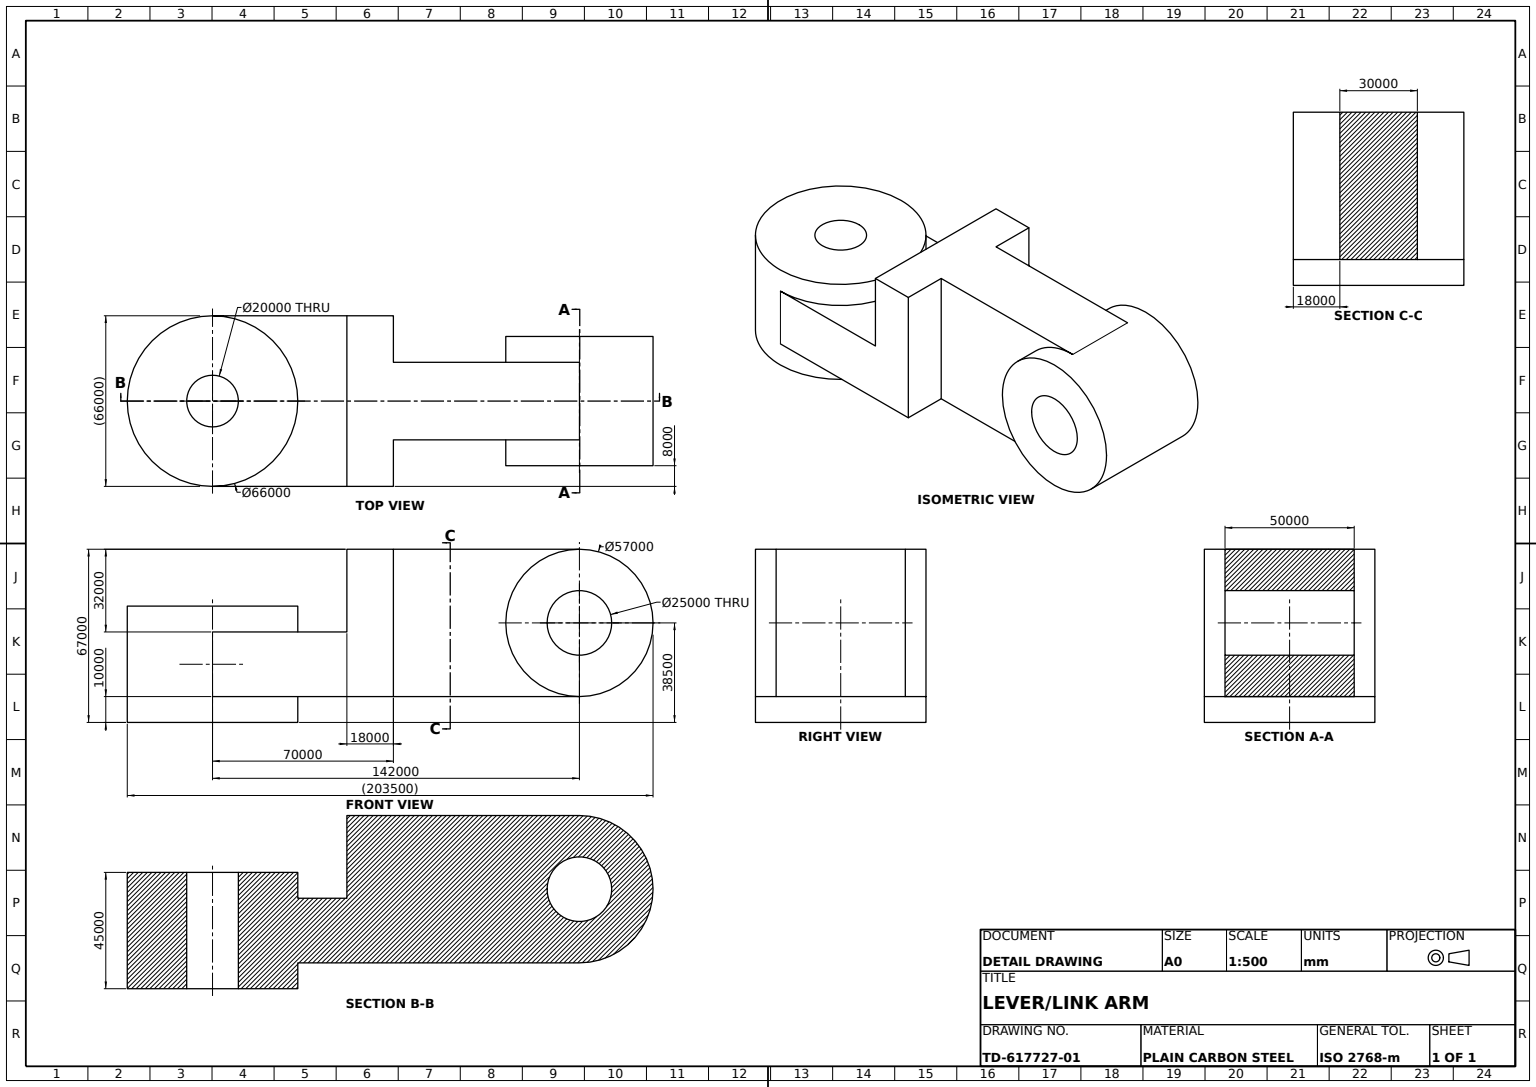
from build123d import *

# Parameters (mm, degrees)
VERTICAL_EYE_BOSS_SKETCH_66_R   = 33000
VERTICAL_EYE_BOSS_66_DEPTH      = 22500
VERTICAL_EYE_BORE_SKETCH_20_R   = 10000
VERTICAL_EYE_BORE_20_DEPTH      = 45000
ARM_BASE_PLATE_DEPTH            = 12500
ARM_WEB_SKETCH_W                = 18000
ARM_WEB_SKETCH_H                = 66000
ARM_WEB_DEPTH                   = 32000
ARM_RIB_PROFILE_SKETCH_W        = 72000
ARM_RIB_PROFILE_SKETCH_H        = 30000
ARM_RIB_DEPTH                   = 57000
HORIZONTAL_EYE_BOSS_SKETCH_R    = 28500
HORIZONTAL_EYE_BOSS_DEPTH       = 25000
HORIZONTAL_EYE_BORE_SKETCH_25_R = 12500
HORIZONTAL_EYE_BORE_25_DEPTH    = 50000


with BuildPart() as part:
    # Vertical Eye Boss Sketch Ø66 → Vertical Eye Boss Ø66 (new, symmetric)
    with BuildSketch(Plane(origin=(0, 0, 0), x_dir=(1, 0, 0), z_dir=(0, 1, 0))):
        with Locations(Location((0, 0, 0), (0, 0, 270))):
            Circle(VERTICAL_EYE_BOSS_SKETCH_66_R)
    extrude(amount=VERTICAL_EYE_BOSS_66_DEPTH, both=True)

    # Vertical Eye Bore Sketch Ø20 → Vertical Eye Bore Ø20 (cut)
    with BuildSketch(Plane(origin=(0, 22500, 0), x_dir=(1, 0, 0), z_dir=(0, 1, 0))):
        with Locations(Location((0, 0, 0), (0, 0, 270))):
            Circle(VERTICAL_EYE_BORE_SKETCH_20_R)
    extrude(amount=-VERTICAL_EYE_BORE_20_DEPTH, mode=Mode.SUBTRACT)

    # Arm Base Sketch → Arm Base Plate (add, symmetric)
    with BuildSketch(Plane(origin=(0, 0, 0), x_dir=(1, 0, 0), z_dir=(0, 1, 0))):
        with BuildLine():
            Line((0, 33000), (70000, 33000))
            Line((70000, 33000), (70000, -33000))
            Line((70000, -33000), (0, -33000))
            ThreePointArc((0, -33000), (33000, 0), (0, 33000))
        make_face()
    extrude(amount=ARM_BASE_PLATE_DEPTH, both=True)

    # Arm Web Sketch → Arm Web (add)
    with BuildSketch(Plane(origin=(0, 12500, 0), x_dir=(1, 0, 0), z_dir=(0, 1, 0))):
        with Locations((61000, 0)):
            Rectangle(ARM_WEB_SKETCH_W, ARM_WEB_SKETCH_H)
    extrude(amount=ARM_WEB_DEPTH)

    # Arm Rib Profile Sketch → Arm Rib (add)
    with BuildSketch(Plane(origin=(0, 44500, 0), x_dir=(1, 0, 0), z_dir=(0, 1, 0))):
        with Locations((106000, 0)):
            Rectangle(ARM_RIB_PROFILE_SKETCH_W, ARM_RIB_PROFILE_SKETCH_H)
    extrude(amount=-ARM_RIB_DEPTH)

    # Horizontal Eye Boss Sketch → Horizontal Eye Boss (add, symmetric)
    with BuildSketch(Plane.XY):
        with Locations((142000, 16000)):
            Circle(HORIZONTAL_EYE_BOSS_SKETCH_R)
    extrude(amount=HORIZONTAL_EYE_BOSS_DEPTH, both=True)

    # Horizontal Eye Bore Sketch Ø25 → Horizontal Eye Bore Ø25 (cut)
    with BuildSketch(Plane.XY.offset(25000)):
        with Locations((142000, 16000)):
            Circle(HORIZONTAL_EYE_BORE_SKETCH_25_R)
    extrude(amount=-HORIZONTAL_EYE_BORE_25_DEPTH, mode=Mode.SUBTRACT)


solid = part.part
